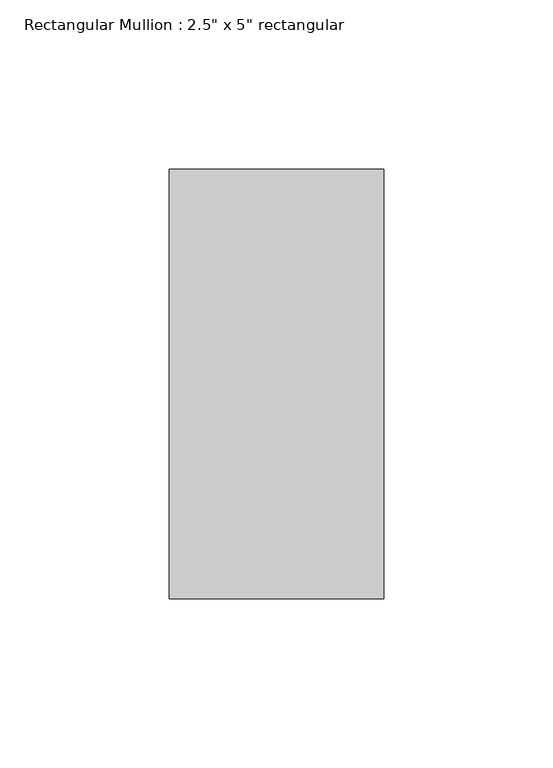
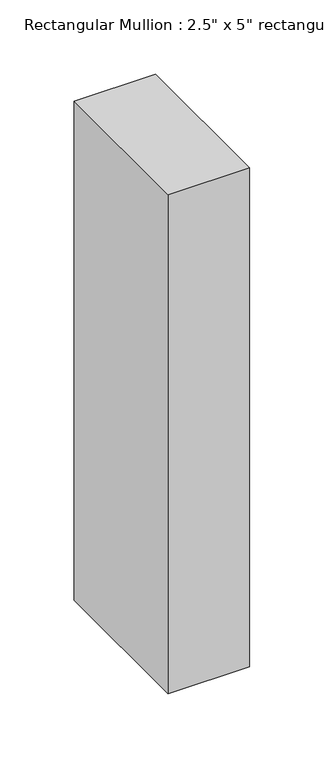
"""IFC4 building model written with IfcOpenShell, lengths in millimetres: member geometry."""

from ifc_helpers import new_model, si_unit, frame, origin, place, context, project, spatial, polyline, outline, extrude, source, transform, mapped, element, save


def member_8b1256c5(model_context):
    return source(origin(), model_context, "Body", "SweptSolid", [
        extrude(outline(polyline([(0.0, 63.5), (0.0, -63.5), (-63.5, -63.5), (-63.5, 63.5), (0.0, 63.5)])), frame((0.0, 0.0, -410.6333333), z_axis=(0.0, 0.0, 1.0), x_axis=(1.0, 0.0, 0.0)), (0.0, 0.0, 1.0), 410.6333333),
    ])


if __name__ == "__main__":
    model = new_model("IFC4")
    model_context = context("Model", 3, world=origin())
    ifc_project = project(units=[si_unit("LENGTHUNIT", "METRE", prefix="MILLI")], contexts=[model_context])
    site = spatial("IfcSite", under=ifc_project)
    building = spatial("IfcBuilding", under=site)
    placement = place(None, origin())
    member_shape = member_8b1256c5(model_context)
    element("IfcMember", 1, ObjectType="Rectangular Mullion : 2.5\" x 5\" rectangular", at=placement, inside=building, context=model_context, shape_type="MappedRepresentation", body=[
        mapped(member_shape, transform((0.0, 0.0, 0.0), x_axis=(1.0, 0.0, 0.0), y_axis=(0.0, 1.0, 0.0), z_axis=(0.0, 0.0, 1.0))),
    ])
    save(model, "model.ifc")

# Revit data of these elements
# Type "Rectangular Mullion : 2.5\" x 5\" rectangular"
#   built-in parameter 1007304 = 0.416667 (stored number, unit not read)
#   built-in parameter 1007301 = 0.104167 (stored number, unit not read)
#   built-in parameter 1007300 = 0.104167 (stored number, unit not read)
